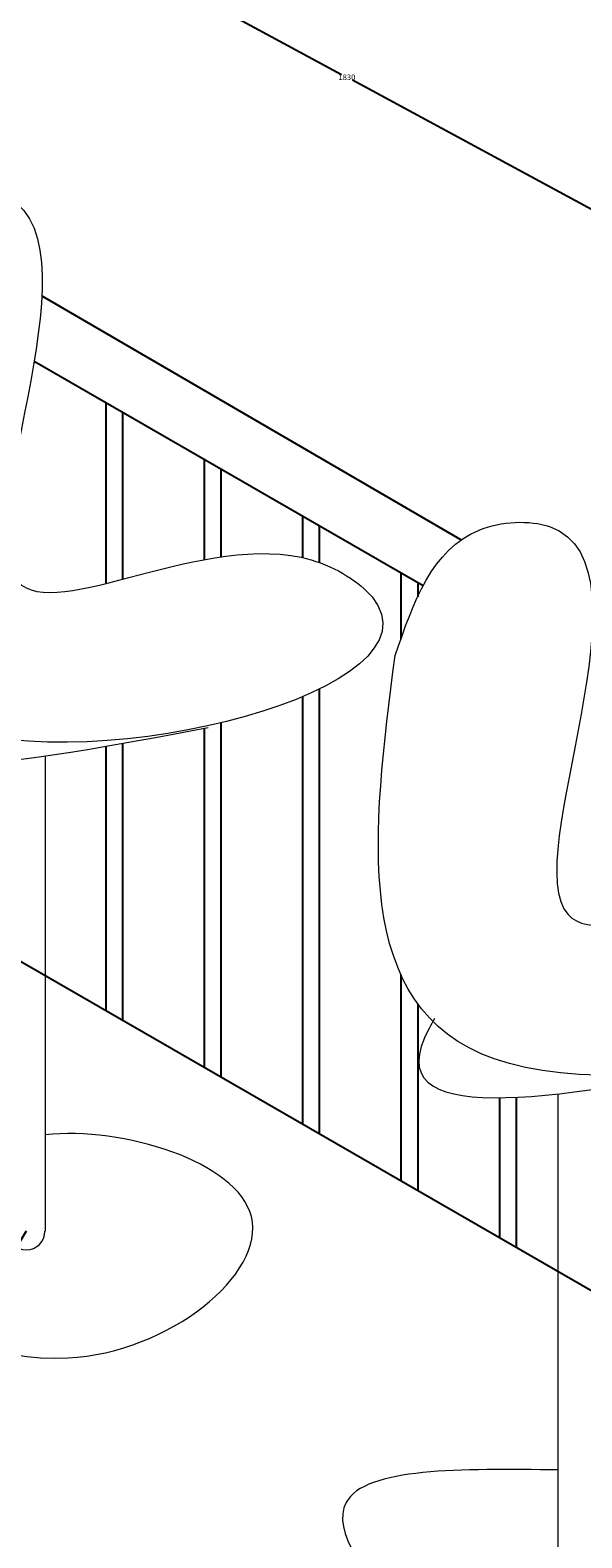
# Model space of a CAD drawing. Units: metres. Extents: x -2391 to 4922, y -635 to 4845.
# Tile 7 of 37: x -1367 to -871, y 53 to 1408. Entities that reach past the tile are written whole.
import ezdxf

# ---------------------------------------------------------------- set-up
doc = ezdxf.new("R2010")
doc.units = ezdxf.units.M
doc.header["$MEASUREMENT"] = 0
for name, color, linetype, lineweight in [('A-ANNO-DIMS', 2, 'Continuous', 18), ('A-FLOR-FIXT', 3, 'Continuous', 25), ('A-FURN', 8, 'Continuous', 18)]:
    doc.layers.add(name, color=color, linetype=linetype, lineweight=lineweight)
doc.styles.get("Standard").update_dxf_attribs({"font": 'arial.ttf'})
doc.dimstyles.get("Standard").update_dxf_attribs({"dimtxt": 5, "dimasz": 4, "dimexe": 0.18, "dimexo": 0.0625, "dimgap": 0.09, "dimtad": 0, "dimtih": 1, "dimtoh": 1, "dimdec": 0, "dimzin": 0, "dimdsep": 46, "dimtxsty": 'Standard', "dimcen": 0.09, "dimadec": 0, "dimazin": 0, "dimtfac": 1, "dimtdec": 0, "dimtofl": 0, "dimtmove": 0, "dimatfit": 3, "dimfxl": 1, "dimtolj": 1, "dimtzin": 0, "dimarcsym": 0})

# ---------------------------------------------------------------- blocks, each defined once
blk = doc.blocks.new('STOOL-BAR')
for p, q in [((193.7, 114.2), (193.7, 537.3)), ((227.2, 541.6), (227.2, 114.2))]:
    blk.add_line(p, q)
blk.add_arc((210.4, 114.2), 16.7, 180, 0)
for points, knots in [([(47.2, 931.3), (26.8, 772.8), (-15.6, 443.8), (639.9, 614.2), (403.7, 766.2), (59.9, 548.3), (308.4, 1061), (87.9, 1049.3), (63.7, 979.1), (47.2, 931.3)], [0, 0, 0, 0, 373.373325, 775.091582, 839.205201, 1103.589215, 1452.822506, 1516.235646, 1651.960559, 1651.960559, 1651.960559, 1651.960559]), ([(82.7, 605.1), (79.4, 599.1), (25.4, 501.4), (205.2, 535.3), (373.8, 567.1)], [0, 0, 0, 0, 19.816883, 320.720948, 320.720948, 320.720948, 320.720948]), ([(193.7, 199.1), (106.9, 200.3), (-113.9, 203.4), (215.4, -95.9), (508.4, 143.5), (296.5, 208.8), (227.2, 200.8)], [0, 0, 0, 0, 131.596892, 334.838301, 476.929251, 613.088937, 613.088937, 613.088937, 613.088937])]:
    blk.add_open_spline(points, degree=3, knots=knots)
blk = doc.blocks.new('*D8')
at = {"layer": 'A-ANNO-DIMS', "color": 0, "lineweight": -2, "transparency": 16777216}
for p, q in [((-2047.3, 3005.2), (-2047.3, -631.4)), ((4577.8, 2350.2), (4577.8, -631.4)), ((-2043.3, -631.2), (1257.6, -631.2)), ((4573.8, -631.2), (1272.8, -631.2))]:
    blk.add_line(p, q, dxfattribs=at)
at = {"layer": 'A-ANNO-DIMS', "color": 0, "transparency": 16777216}
for points in [[(-2043.3, -630.6), (-2043.3, -631.9), (-2047.3, -631.2)], [(4573.8, -630.6), (4573.8, -631.9), (4577.8, -631.2)]]:
    blk.add_solid(points, dxfattribs=at)
at = {"layer": 'Defpoints', "color": 0, "transparency": 16777216}
for p in [(-2047.3, 3005.3), (4577.8, 2350.3), (4577.8, -631.2)]:
    blk.add_point(p, dxfattribs=at)
at = {"layer": 'A-ANNO-DIMS', "color": 0, "transparency": 16777216, "insert": (1265.2, -631.2), "char_height": 5, "attachment_point": 5}
blk.add_mtext('\\A1;6625', dxfattribs=at)
blk = doc.blocks.new('*D10')
at = {"layer": 'A-ANNO-DIMS', "color": 0, "lineweight": -2, "transparency": 16777216}
for p, q in [((550.7, 4505.3), (-2384, 4505.3)), ((-2383.8, 4501.3), (-2383.8, 2107.9)), ((-2383.8, -290.7), (-2383.8, 2102.6)), ((-488.6, -294.7), (-2384, -294.7))]:
    blk.add_line(p, q, dxfattribs=at)
at = {"layer": 'A-ANNO-DIMS', "color": 0, "transparency": 16777216}
for points in [[(-2384.5, 4501.3), (-2383.2, 4501.3), (-2383.8, 4505.3)], [(-2384.5, -290.7), (-2383.2, -290.7), (-2383.8, -294.7)]]:
    blk.add_solid(points, dxfattribs=at)
at = {"layer": 'Defpoints', "color": 0, "transparency": 16777216}
for p in [(-2383.8, 4505.3), (550.7, 4505.3), (-488.5, -294.7)]:
    blk.add_point(p, dxfattribs=at)
at = {"layer": 'A-ANNO-DIMS', "color": 0, "transparency": 16777216, "insert": (-2383.8, 2105.3), "char_height": 5, "attachment_point": 5}
blk.add_mtext('\\A1;4800', dxfattribs=at)
blk = doc.blocks.new('*D46')
at = {"layer": 'A-ANNO-DIMS', "color": 0, "lineweight": -2, "transparency": 16777216}
for p, q in [((-2047.3, 1505.3), (-1887.1, 1801.4)), ((-1883.7, 1799.3), (-1087.4, 1368.5)), ((-281.2, 932.4), (-1077.6, 1363.2)), ((-437.8, 634.6), (-277.6, 930.6))]:
    blk.add_line(p, q, dxfattribs=at)
at = {"layer": 'A-ANNO-DIMS', "color": 0, "transparency": 16777216}
for points in [[(-1883.4, 1799.9), (-1884, 1798.7), (-1887.2, 1801.2)], [(-280.9, 933), (-281.6, 931.8), (-277.7, 930.5)]]:
    blk.add_solid(points, dxfattribs=at)
at = {"layer": 'Defpoints', "color": 0, "transparency": 16777216}
for p in [(-2047.3, 1505.3), (-277.7, 930.5), (-437.8, 634.5)]:
    blk.add_point(p, dxfattribs=at)
at = {"layer": 'A-ANNO-DIMS', "color": 0, "transparency": 16777216, "insert": (-1082.5, 1365.9), "char_height": 5, "attachment_point": 5}
blk.add_mtext('\\A1;1830', dxfattribs=at)
blk = doc.blocks.new('*D51')
at = {"layer": 'A-ANNO-DIMS', "color": 0, "lineweight": -2, "transparency": 16777216}
for p, q in [((-1370.5, 328.3), (-1544.9, 40.4)), ((-1541.4, 38.4), (-1301.9, -106.6)), ((-876, 28.7), (-1050.4, -259.2)), ((-1053.8, -257), (-1293.2, -111.9))]:
    blk.add_line(p, q, dxfattribs=at)
at = {"layer": 'A-ANNO-DIMS', "color": 0, "transparency": 16777216}
for points in [[(-1541.1, 39), (-1541.8, 37.9), (-1544.8, 40.5)], [(-1053.4, -256.4), (-1054.1, -257.5), (-1050.3, -259)]]:
    blk.add_solid(points, dxfattribs=at)
at = {"layer": 'Defpoints', "color": 0, "transparency": 16777216}
for p in [(-1370.5, 328.3), (-1544.8, 40.5), (-876, 28.8)]:
    blk.add_point(p, dxfattribs=at)
at = {"layer": 'A-ANNO-DIMS', "color": 0, "transparency": 16777216, "insert": (-1297.6, -109.3), "char_height": 5, "attachment_point": 5}
blk.add_mtext('\\A1;578.1', dxfattribs=at)

msp = doc.modelspace()

# ---------------------------------------------------------------- linework, layer by layer
at = {"layer": 'A-FLOR-FIXT'}
for p, q in [((-1356.5795, 1169.3703), (-979.7857, 950.0161)), ((-1013.9995, 908.6801), (-1363.5091, 1110.4696)), ((-1299.1098, 1073.2887), (-1299.1098, 910.7494)), ((-1284.1017, 1064.6237), (-1284.1017, 914.5591)), ((-1210.7084, 1022.25), (-1210.7084, 932.1822)), ((-1195.7003, 1013.5851), (-1195.7003, 934.679)), ((-1122.3069, 971.2114), (-1122.3069, 933.9607)), ((-1107.2988, 962.5465), (-1107.2988, 929.5902)), ((-1033.9055, 920.1728), (-1033.9055, 860.9553)), ((-1018.8974, 911.5079), (-1018.8974, 898.8128)), ((-1107.2988, 815.8513), (-1107.2988, 416.1357)), ((-1122.3069, 808.9983), (-1122.3069, 424.8006)), ((-1741.1171, 782.0708), (-488.4886, 58.8654)), ((-1210.7084, 780.553), (-1210.7084, 475.8392)), ((-1195.7003, 785.4036), (-1195.7003, 467.1743)), ((-1299.1098, 764.3687), (-1299.1098, 526.8778)), ((-1284.1017, 766.9948), (-1284.1017, 518.2129)), ((-1033.9055, 558.7925), (-1033.9055, 373.762)), ((-1018.8974, 532.8725), (-1018.8974, 365.0971)), ((-945.504, 448.3612), (-945.504, 322.7234)), ((-930.4959, 448.7924), (-930.4959, 314.0584))]:
    msp.add_line(p, q, dxfattribs=at)

# ---------------------------------------------------------------- block references
at = {"layer": 'A-FURN'}
for p in [(-1580.882, 214.116), (-1086.3941, -85.4426)]:
    msp.add_blockref('STOOL-BAR', p, dxfattribs=at)

# ---------------------------------------------------------------- dimensions: what is measured, and where the dimension line sits
at = {"layer": 'A-ANNO-DIMS'}
for base, p1, p2, angle, override, picture, middle in [((-2383.8343, 4505.2763), (-488.4886, -294.7237), (550.7419, 4505.2763), 90, {"dimdec": 0, "dimlfac": 1, "dimrnd": 0, "dimzin": 0, "dimdsep": 46, "dimlunit": 2}, '*D10', (-2383.8343, 2105.2763)), ((-277.7211, 930.4802), (-2047.3343, 1505.2763), (-437.841, 634.5176), 331.5859855, {"dimdec": 0, "dimlfac": 1, "dimrnd": 0, "dimzin": 0, "dimdsep": 46, "dimlunit": 2}, '*D46', (-1082.4677, 1365.8595)), ((-1544.828, 40.5209), (-875.9874, 28.7702), (-1370.4753, 328.3288), 148.7927031, {"dimdec": 1, "dimlfac": 1, "dimrnd": 0, "dimzin": 0, "dimdsep": 46, "dimlunit": 2}, '*D51', (-1297.5841, -109.2584))]:
    dim = msp.add_linear_dim(base=base, p1=p1, p2=p2, angle=angle, dimstyle='Standard', override=override, dxfattribs=at)
    dim.commit()
    dim.dimension.update_dxf_attribs({"geometry": picture, "text_midpoint": middle})
dim = msp.add_linear_dim(base=(4577.76, -631.2237), p1=(-2047.3343, 3005.2763), p2=(4577.76, 2350.2763), dimstyle='Standard', override={"dimdec": 0, "dimlfac": 1, "dimrnd": 0, "dimzin": 0, "dimdsep": 46, "dimlunit": 2}, dxfattribs=at)
dim.commit()
dim.dimension.update_dxf_attribs({"geometry": '*D8', "text_midpoint": (1265.2128, -631.2237)})

doc.saveas('drawing.dxf')
